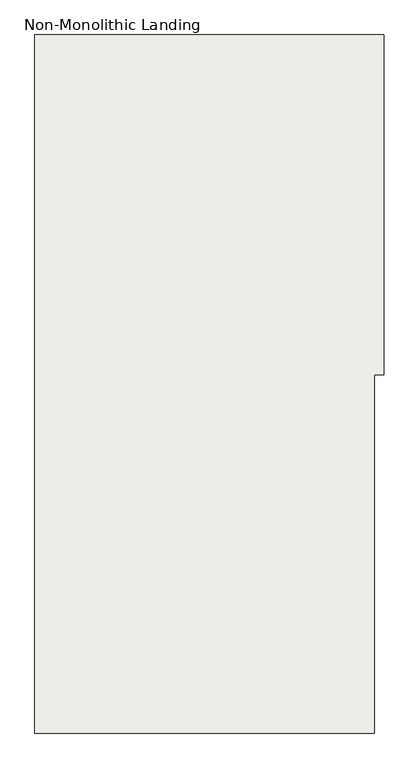
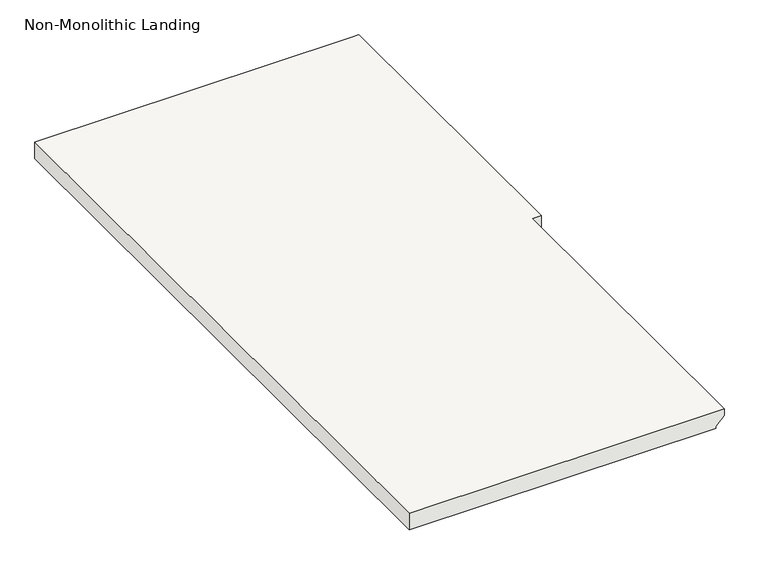
"""IFC4 building model written with IfcOpenShell, lengths in millimetres: slab geometry, Non-Monolithic Landing."""

from ifc_helpers import new_model, si_unit, origin, place, context, project, spatial, faceted_brep, source, transform, mapped, element, save


def non_monolithic_landing_e910b983(model_context):
    return source(origin(), model_context, "Body", "Brep", [
        faceted_brep([(-6548.9591614, -543.1950563, 4781.55), (-6574.3591614, -543.1950563, 4756.15), (-6574.3591614, 371.2049437, 4756.15), (-6548.9591614, 371.2049437, 4781.55), (-6548.9591614, 421.4825188, 4800.6), (-6523.5591614, 421.4825188, 4800.6), (-6523.5591614, 1335.8825188, 4800.6), (-6548.9591614, 1335.8825188, 4800.6), (-7463.3591614, 1335.8825188, 4800.6), (-7463.3591614, -543.1950563, 4800.6), (-6548.9591614, -543.1950563, 4800.6), (-6574.3591614, 371.2049437, 4749.8), (-6574.3591614, -543.1950563, 4749.8), (-7463.3591614, -543.1950563, 4749.8), (-7463.3591614, 1335.8825188, 4749.8), (-6548.9591614, 1335.8825188, 4749.8), (-6523.5591614, 1335.8825188, 4749.8), (-6523.5591614, 421.4825188, 4749.8), (-6548.9591614, 421.4825188, 4749.8), (-6548.9591614, 371.2049437, 4749.8)], [[[0, 1, 2, 3]], [[4, 5, 6, 7, 8, 9, 10]], [[11, 12, 13, 14, 15, 16, 17, 18, 19]], [[12, 11, 2, 1]], [[11, 19, 3, 2]], [[4, 10, 0, 3, 19, 18]], [[5, 4, 18, 17]], [[6, 5, 17, 16]], [[7, 6, 16, 15]], [[8, 7, 15, 14]], [[9, 8, 14, 13]], [[10, 9, 13, 12, 1, 0]]]),
    ])


if __name__ == "__main__":
    model = new_model("IFC4")
    model_context = context("Model", 3, world=origin())
    ifc_project = project(units=[si_unit("LENGTHUNIT", "METRE", prefix="MILLI")], contexts=[model_context])
    site = spatial("IfcSite", under=ifc_project)
    building = spatial("IfcBuilding", under=site)
    placement = place(None, origin())
    non_monolithic_landing_shape = non_monolithic_landing_e910b983(model_context)
    element("IfcSlab", 1, ObjectType="Non-Monolithic Landing", at=placement, inside=building, context=model_context, shape_type="MappedRepresentation", body=[
        mapped(non_monolithic_landing_shape, transform((0.0, 0.0, 0.0), x_axis=(1.0, 0.0, 0.0), y_axis=(0.0, 1.0, 0.0), z_axis=(0.0, 0.0, 1.0))),
    ])
    save(model, "model.ifc")
